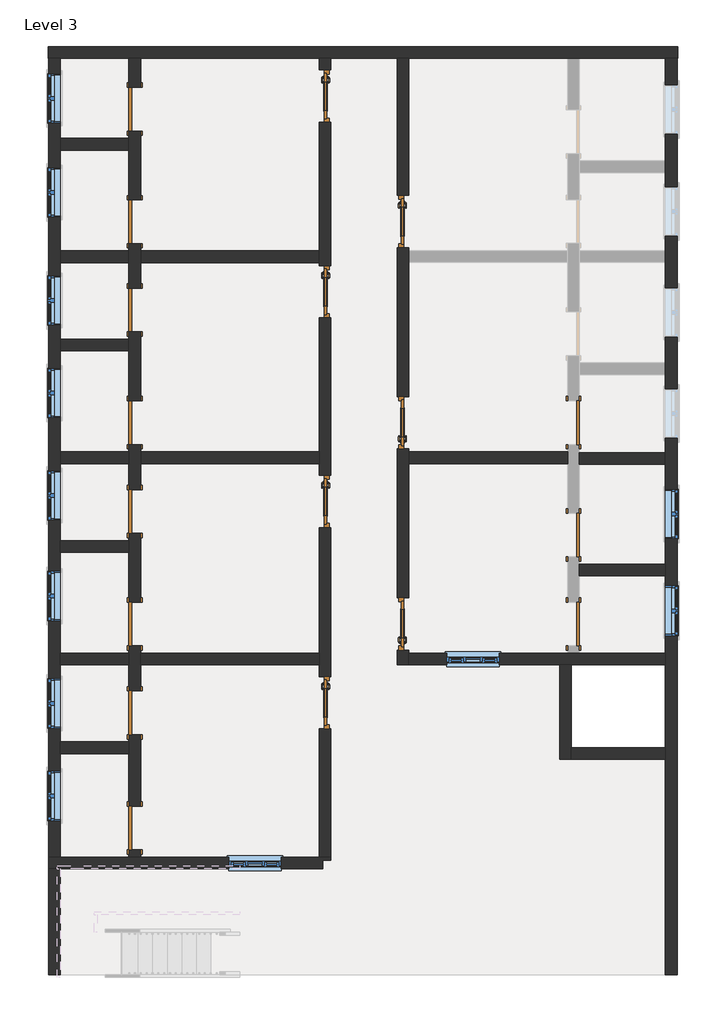
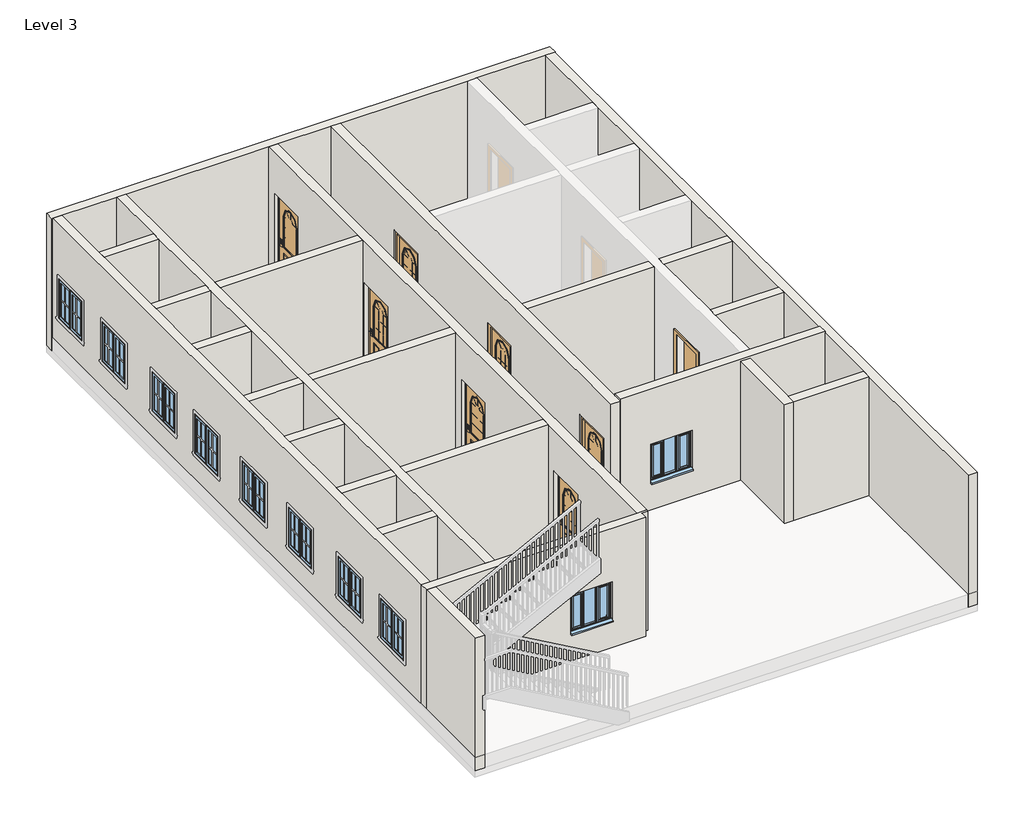
# One storey, part 1 of 4: 24 walls, 18 doors, 12 windows.
# Revit data of these elements (continued)
# Element 41 (IfcWall, "9\" w") (continued)
#   Materials on its faces: "Default Wall", "Wood - Stained"
# Element 42 (IfcWall, "9\" w")
#   Top Offset = 0' - 0"
#   Base Offset = 0' - 0"
#   wall height = 10' - 0"
#   Phase Created = New Construction
#   Base Constraint = Level 3
#   Top Constraint = Level 4
#   Materials on its faces: "Default Wall", "Wood - Stained", "Earth"
# Element 43 (IfcWindow, "Window-Casement-Double : 34\" x 36\"")
#   Mark = "33"
#   Window Inset = 0' - 0"
#   Interior Wall Closure = 0' - 2 1/4"
#   Frame Extension = 0' - 0 1/4"
#   Exterior Wall Closure = 0' - 1 1/4"
#   Interior Trim Visibility = yes
#   Exterior Trim Visibility = yes
#   Phase Created = New Construction
#   Materials on its faces: "Wood - Stained", "Glass", "Clad - White"
# Element 44 (IfcWindow, "Window-Casement-Double : 34\" x 36\"")
#   Mark = "34"
#   Window Inset = 0' - 0"
#   Interior Wall Closure = 0' - 2 1/4"
#   Frame Extension = 0' - 0 1/4"
#   Exterior Wall Closure = 0' - 1 1/4"
#   Interior Trim Visibility = yes
#   Exterior Trim Visibility = yes
#   Phase Created = New Construction
#   Materials on its faces: "Wood - Stained", "Glass", "Clad - White"
# Element 45 (IfcWindow, "Window-Casement-Double : 34\" x 36\"")
#   Mark = "35"
#   Window Inset = 0' - 0"
#   Interior Wall Closure = 0' - 2 1/4"
#   Frame Extension = 0' - 0 1/4"
#   Exterior Wall Closure = 0' - 1 1/4"
#   Interior Trim Visibility = yes
#   Exterior Trim Visibility = yes
#   Phase Created = New Construction
#   Materials on its faces: "Wood - Stained", "Glass", "Clad - White"
# Element 46 (IfcWindow, "Window-Casement-Double : 34\" x 36\"")
#   Mark = "36"
#   Window Inset = 0' - 0"
#   Interior Wall Closure = 0' - 2 1/4"
#   Frame Extension = 0' - 0 1/4"
#   Exterior Wall Closure = 0' - 1 1/4"
#   Interior Trim Visibility = yes
#   Exterior Trim Visibility = yes
#   Phase Created = New Construction
#   Materials on its faces: "Wood - Stained", "Glass", "Clad - White"
# Element 47 (IfcWindow, "Window-Casement-Double : 34\" x 36\"")
#   Mark = "37"
#   Window Inset = 0' - 0"
#   Interior Wall Closure = 0' - 2 1/4"
#   Frame Extension = 0' - 0 1/4"
#   Exterior Wall Closure = 0' - 1 1/4"
#   Interior Trim Visibility = yes
#   Exterior Trim Visibility = yes
#   Phase Created = New Construction
#   Materials on its faces: "Wood - Stained", "Glass", "Clad - White"
# Element 48 (IfcWindow, "Window-Casement-Double : 34\" x 36\"")
#   Mark = "38"
#   Window Inset = 0' - 0"
#   Interior Wall Closure = 0' - 2 1/4"
#   Frame Extension = 0' - 0 1/4"
#   Exterior Wall Closure = 0' - 1 1/4"
#   Interior Trim Visibility = yes
#   Exterior Trim Visibility = yes
#   Phase Created = New Construction
#   Materials on its faces: "Wood - Stained", "Glass", "Clad - White"
# Element 49 (IfcWindow, "Window-Casement-Double : 34\" x 36\"")
#   Mark = "39"
#   Window Inset = 0' - 0"
#   Interior Wall Closure = 0' - 2 1/4"
#   Frame Extension = 0' - 0 1/4"
#   Exterior Wall Closure = 0' - 1 1/4"
#   Interior Trim Visibility = yes
#   Exterior Trim Visibility = yes
#   Phase Created = New Construction
#   Materials on its faces: "Wood - Stained", "Glass", "Clad - White"
# Element 50 (IfcWindow, "Window-Casement-Double : 34\" x 36\"")
#   Mark = "40"
#   Window Inset = 0' - 0"
#   Interior Wall Closure = 0' - 2 1/4"
#   Frame Extension = 0' - 0 1/4"
#   Exterior Wall Closure = 0' - 1 1/4"
#   Interior Trim Visibility = yes
#   Exterior Trim Visibility = yes
#   Phase Created = New Construction
#   Materials on its faces: "Wood - Stained", "Glass", "Clad - White"
# Element 51 (IfcWindow, "Window-Casement-Double : 34\" x 36\"")
#   Mark = "41"
#   Window Inset = 0' - 0"
#   Interior Wall Closure = 0' - 2 1/4"
#   Frame Extension = 0' - 0 1/4"
#   Exterior Wall Closure = 0' - 1 1/4"
#   Interior Trim Visibility = yes
#   Exterior Trim Visibility = yes
#   Phase Created = New Construction
#   Materials on its faces: "Wood - Stained", "Glass", "Clad - White"
# Element 52 (IfcWindow, "Window-Casement-Double : 34\" x 36\"")
#   Mark = "42"
#   Window Inset = 0' - 0"
#   Interior Wall Closure = 0' - 2 1/4"
#   Frame Extension = 0' - 0 1/4"
#   Exterior Wall Closure = 0' - 1 1/4"
#   Interior Trim Visibility = yes
#   Exterior Trim Visibility = yes
#   Phase Created = New Construction
#   Materials on its faces: "Wood - Stained", "Glass", "Clad - White"
# Element 53 (IfcWindow, "Windows_Tpl_Plain : 910x910mm")
#   Mark = "47"
#   Phase Created = New Construction
#   Materials on its faces: "Window Frame", "Glass"
# Element 54 (IfcWindow, "Windows_Tpl_Plain : 910x910mm")
#   Mark = "48"
#   Phase Created = New Construction
#   Materials on its faces: "Window Frame", "Glass"
# Materials
#   "Door - Glazing": colour RGB 0 0 255, transparency 0.75
#   "Door - Panel": class "Wood", colour RGB 210 159 95, transparency 0, Cost = 0
#   "Door - Frame/Mullion": class "Wood", colour RGB 212 179 113, transparency 0
#   "Door - Handle": colour RGB 247 247 247, transparency 0
#   "Door - Frame": colour RGB 118 70 51, transparency 0, Cost = 0
#   "Wood - Stained": class "Wood", colour RGB 224 178 126, transparency 0, Cost = 0
#   "Glass": class "Glass", colour RGB 0 128 192, transparency 0.75, Description = "Soda Lime Glass", Cost = 0
#   "Clad - White": class "Wood", colour RGB 242 242 238, transparency 0, Cost = 0
#   "Window Frame": colour RGB 249 249 249, transparency 0
#   "Default Wall": colour RGB 128 128 128, transparency 0, Cost = 0
#   "Brick, Common": class "Masonry", colour RGB 170 98 104, transparency 0, Description = "Common brick", Cost = 0
#   "Phase-Exist": colour RGB 127 127 127, transparency 0, Cost = 0
#   "Doors - Glazing Bars": colour RGB 158 107 65, transparency 0
#   "Cherry": class "Wood", colour RGB 226 177 128, transparency 0, Description = "Prunus Serotina", Cost = 0
#   "Door - Architrave": class "Wood", colour RGB 154 90 5, transparency 0
#   "Earth": class "Generic", colour RGB 97 75 62, transparency 0, Description = "Soil", Cost = 0
